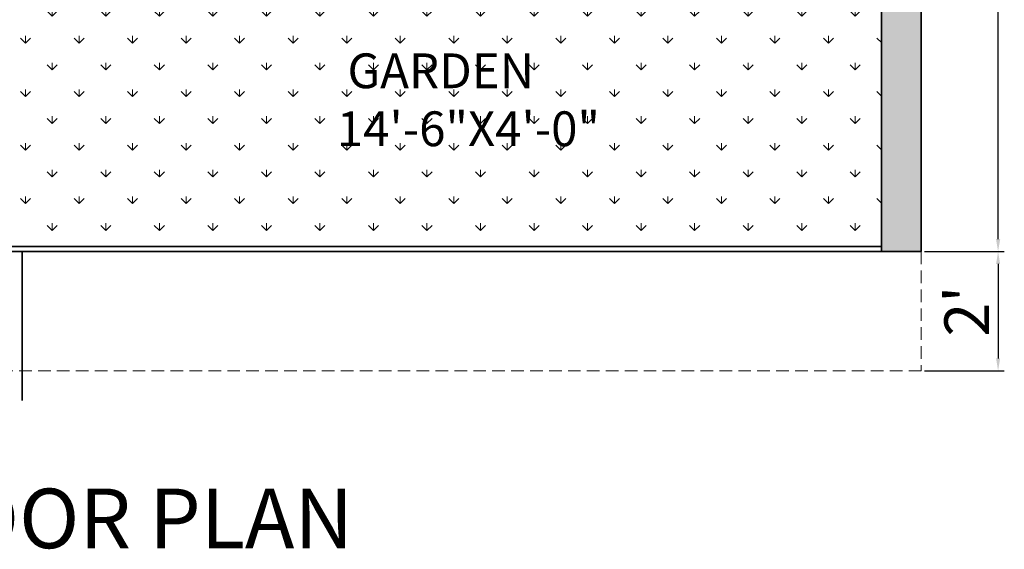
# Model space of a CAD drawing. Units: inches. Extents: x 1566 to 2546, y 1087 to 2705.
# Tile 2 of 27: x 1820 to 2018, y 1094 to 1201. Entities that reach past the tile are written whole.
import ezdxf

# ---------------------------------------------------------------- set-up
doc = ezdxf.new("R2010")
doc.units = ezdxf.units.IN
doc.linetypes.add('DASHED', pattern=[19.05, 12.7, -6.35])
for name, color, linetype, lineweight in [('A-ANNO-DIMS', 2, 'Continuous', 18), ('A-AREA-IDEN', 7, 'Continuous', 18), ('A-FLOR-OVHD', 8, 'DASHED', 18), ('A-FLOR-PATT', 3, 'Continuous', 13), ('A-WALL', 7, 'Continuous', 35), ('A-WALL-PATT', 8, 'Continuous', 13)]:
    doc.layers.add(name, color=color, linetype=linetype, lineweight=lineweight)
doc.styles.get("Standard").update_dxf_attribs({"font": 'arial.ttf'})
doc.dimstyles.new('ISO-25', dxfattribs={"dimtxt": 2.5, "dimasz": 2.5, "dimexe": 1.25, "dimexo": 0.625, "dimtad": 1, "dimtxsty": 'Standard', "dimcen": 2.5, "dimadec": 0, "dimazin": 0, "dimtfac": 1, "dimtmove": 0, "dimatfit": 3, "dimfxl": 1, "dimarcsym": 0})

# ---------------------------------------------------------------- blocks, each defined once
blk = doc.blocks.new('*D7')
at = {"layer": 'A-ANNO-DIMS', "color": 0, "lineweight": -2, "transparency": 16777216}
for p, q in [((2002.15, 1778.2), (2018.24, 1778.2)), ((2016.99, 1156.7), (2016.99, 1775.7)), ((2002.15, 1154.2), (2018.24, 1154.2))]:
    blk.add_line(p, q, dxfattribs=at)
at = {"layer": 'A-ANNO-DIMS', "color": 0, "transparency": 16777216}
for points in [[(2016.58, 1775.7), (2017.41, 1775.7), (2016.99, 1778.2)], [(2016.58, 1156.7), (2017.41, 1156.7), (2016.99, 1154.2)]]:
    blk.add_solid(points, dxfattribs=at)
at = {"layer": 'Defpoints', "color": 0, "transparency": 16777216}
for p in [(2001.53, 1778.2), (2016.99, 1778.2), (2001.53, 1154.2)]:
    blk.add_point(p, dxfattribs=at)
at = {"layer": 'A-ANNO-DIMS', "color": 0, "transparency": 16777216, "insert": (2011.77, 1466.2), "char_height": 9, "attachment_point": 5, "rotation": 90}
blk.add_mtext("52'", dxfattribs=at)
blk = doc.blocks.new('*D11')
at = {"layer": 'A-ANNO-DIMS', "color": 0, "lineweight": -2, "transparency": 16777216}
for p, q in [((2002.15, 1154.2), (2018.24, 1154.2)), ((2016.99, 1151.7), (2016.99, 1132.7)), ((2002.15, 1130.2), (2018.24, 1130.2))]:
    blk.add_line(p, q, dxfattribs=at)
at = {"layer": 'A-ANNO-DIMS', "color": 0, "transparency": 16777216}
for points in [[(2016.58, 1151.7), (2017.41, 1151.7), (2016.99, 1154.2)], [(2016.58, 1132.7), (2017.41, 1132.7), (2016.99, 1130.2)]]:
    blk.add_solid(points, dxfattribs=at)
at = {"layer": 'Defpoints', "color": 0, "transparency": 16777216}
for p in [(2001.53, 1154.2), (2001.53, 1130.2), (2016.99, 1130.2)]:
    blk.add_point(p, dxfattribs=at)
at = {"layer": 'A-ANNO-DIMS', "color": 0, "transparency": 16777216, "insert": (2011.85, 1142.2), "char_height": 9, "attachment_point": 5, "rotation": 90}
blk.add_mtext("2'", dxfattribs=at)

msp = doc.modelspace()

# ---------------------------------------------------------------- hatches: boundary and pattern name
at = {"layer": 'A-FLOR-PATT'}
h = msp.add_hatch(dxfattribs=at)
h.set_pattern_fill('GRASS', color=256, scale=0.3)
h.paths.add_polyline_path([(1745.53, 1270.2), (1645.53, 1270.2), (1645.53, 1159.2), (1745.53, 1159.2)])
h.paths.add_polyline_path([(1993.53, 1203.2), (1819.53, 1203.2), (1819.53, 1155.2), (1993.53, 1155.2)])
h.paths.add_polyline_path([(1667.62, 1196.42), (1716.72, 1196.42), (1716.72, 1222.54), (1667.62, 1222.54)], flags=24)
h.paths.add_polyline_path([(1881.06, 1171.45), (1935.47, 1171.45), (1935.47, 1197.57), (1881.06, 1197.57)], flags=24)
at = {"layer": 'A-WALL-PATT'}
h = msp.add_hatch(color=256, dxfattribs=at)
h.dxf.hatch_style = 1
h.paths.add_polyline_path([(2001.53, 1778.2), (1641.53, 1778.2), (1641.53, 1746.2), (1649.53, 1746.2), (1649.53, 1770.2), (1769.53, 1770.2), (1769.53, 1650.2), (1767.53, 1650.2), (1767.53, 1648.2), (1767.53, 1646.2), (1819.53, 1646.2), (1819.53, 1650.2), (1773.53, 1650.2), (1773.53, 1770.2), (1941.53, 1770.2), (1941.53, 1756.2), (1945.53, 1756.2), (1945.53, 1770.2), (1993.53, 1770.2), (1993.53, 1650.2), (1945.53, 1650.2), (1945.53, 1652.2), (1943.53, 1652.2), (1941.53, 1652.2), (1941.53, 1650.2), (1867.53, 1650.2), (1867.53, 1642.2), (1871.53, 1642.2), (1871.53, 1646.2), (1993.53, 1646.2), (1993.53, 1526.2), (1871.53, 1526.2), (1871.53, 1606.2), (1867.53, 1606.2), (1867.53, 1522.2), (1993.53, 1522.2), (1993.53, 1387.2), (1959.53, 1387.2), (1959.53, 1397.2), (1955.53, 1397.2), (1955.53, 1387.2), (1903.53, 1387.2), (1903.53, 1383.2), (1993.53, 1383.2), (1993.53, 1364.3), (1993.53, 1211.2), (1939.53, 1211.2), (1939.53, 1203.2), (1993.53, 1203.2), (1993.53, 1154.2), (2001.53, 1154.2)])
h.paths.add_polyline_path([(1649.53, 1646.2), (1731.53, 1646.2), (1731.53, 1650.2), (1649.53, 1650.2), (1649.53, 1674.2), (1641.53, 1674.2), (1641.53, 1622.2), (1649.53, 1622.2)], flags=17)
h.paths.add_polyline_path([(1649.53, 1550.2), (1641.53, 1550.2), (1641.53, 1510.2), (1649.53, 1510.2), (1649.53, 1522.2), (1731.53, 1522.2), (1731.53, 1500.2), (1735.53, 1500.2), (1735.53, 1522.2), (1767.53, 1522.2), (1767.53, 1500.2), (1771.53, 1500.2), (1771.53, 1526.2), (1649.53, 1526.2)], flags=17)
h.paths.add_polyline_path([(1649.53, 1464.2), (1735.53, 1464.2), (1735.53, 1470.2), (1731.53, 1470.2), (1731.53, 1468.2), (1649.53, 1468.2), (1649.53, 1480.2), (1641.53, 1480.2), (1641.53, 1419.2), (1649.53, 1419.2)], flags=17)
h.paths.add_polyline_path([(1649.53, 1323.2), (1641.53, 1323.2), (1641.53, 1270.2), (1667.53, 1270.2), (1667.53, 1278.2), (1649.53, 1278.2)], flags=17)
h.paths.add_polyline_path([(1763.53, 1278.2), (1727.53, 1278.2), (1727.53, 1270.2), (1763.53, 1270.2)], flags=17)
h.paths.add_polyline_path([(1823.53, 1383.2), (1827.53, 1383.2), (1827.53, 1385.2), (1827.53, 1387.2), (1819.53, 1387.2), (1819.53, 1324.21), (1819.53, 1278.2), (1811.53, 1278.2), (1811.53, 1274.2), (1811.53, 1270.2), (1819.53, 1270.2), (1819.53, 1203.2), (1877.53, 1203.2), (1877.53, 1211.2), (1823.53, 1211.2)], flags=17)

# ---------------------------------------------------------------- linework, layer by layer
at = {"layer": 'A-FLOR-OVHD', "ltscale": 0.2}
for p, q in [((2001.53, 1154.2), (2001.53, 1130.2)), ((2001.53, 1130.2), (1605.53, 1130.2))]:
    msp.add_line(p, q, dxfattribs=at)
at = {"layer": 'A-WALL'}
for p, q in [((2001.53, 1778.2), (2001.53, 1154.2)), ((1993.53, 1203.2), (1993.53, 1154.2)), ((2001.53, 1154.2), (1641.53, 1154.2)), ((1993.53, 1155.2), (1745.53, 1155.2)), ((1820.53, 1154.2), (1820.53, 1124.2))]:
    msp.add_line(p, q, dxfattribs=at)

# ---------------------------------------------------------------- texts
at = {"layer": 'A-AREA-IDEN', "attachment_point": 1}
for s, width, insert, char_height in [(' GARDEN\\P14\'-6"X4\'-0"', 111.7553, (1883.88, 1194.09), 7), ('GROUND FLOOR PLAN', 267.5424, (1717.44, 1106.48), 12)]:
    msp.add_mtext_dynamic_manual_height_columns(s, width=width, gutter_width=12.5, heights=[0], dxfattribs=dict(at, insert=insert, char_height=char_height))

# ---------------------------------------------------------------- dimensions: what is measured, and where the dimension line sits
at = {"layer": 'A-ANNO-DIMS'}
for base, p2, picture, middle in [((2016.99, 1778.2), (2001.53, 1778.2), '*D7', (2011.77, 1466.2)), ((2016.99, 1130.2), (2001.53, 1130.2), '*D11', (2011.85, 1142.2))]:
    dim = msp.add_linear_dim(base=base, p1=(2001.53, 1154.2), p2=p2, angle=90, dimstyle='ISO-25', override={"dimtxt": 9, "dimdec": 1, "dimlunit": 3, "dimclrd": 0, "dimclre": 0, "dimclrt": 0, "dimtdec": 1}, dxfattribs=at)
    dim.commit()
    dim.dimension.update_dxf_attribs({"geometry": picture, "text_midpoint": middle})

doc.saveas('drawing.dxf')
